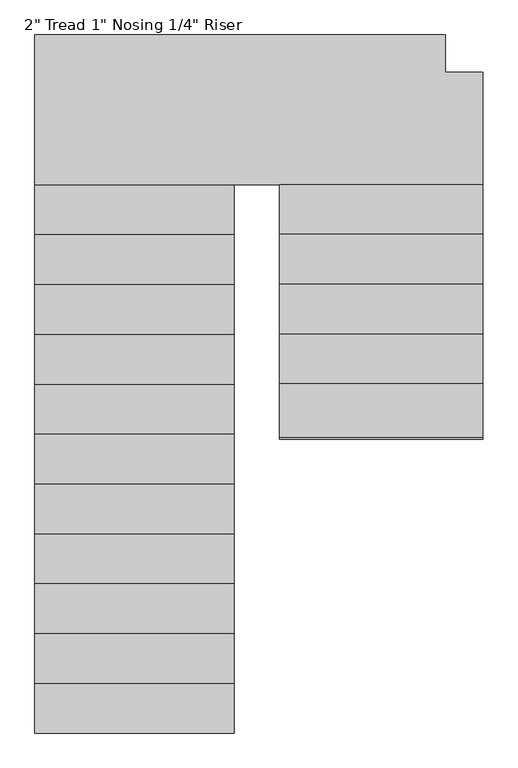
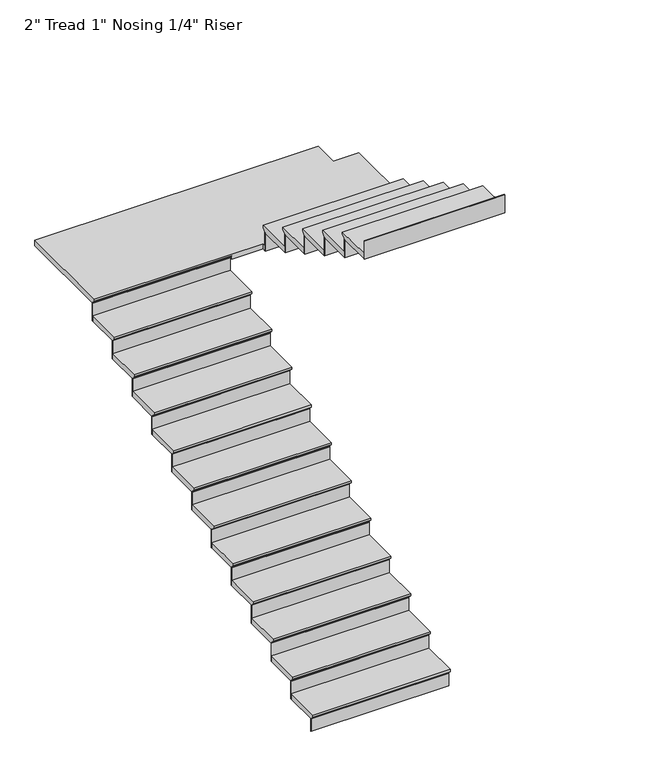
"""IFC4 building model written with IfcOpenShell, lengths in millimetres: stair flight geometry."""

from ifc_helpers import new_model, si_unit, origin, place, context, project, spatial, faceted_brep, source, transform, mapped, element, save


def stair_flight_255c1e55(model_context):
    return source(origin(), model_context, "Body", "Brep", [
        faceted_brep([(-1810.3456086, -4300.9794704, 455.0833333), (-1810.3456086, -4300.9794704, 474.1333333), (-3029.5456086, -4300.9794704, 474.1333333), (-3029.5456086, -4300.9794704, 455.0833333), (-1810.3456086, -4275.5794704, 429.6833333), (-3029.5456086, -4275.5794704, 429.6833333), (-1810.3456086, -3970.7794704, 474.1333333), (-3029.5456086, -3970.7794704, 474.1333333), (-3029.5456086, -4275.5794704, 423.3333333), (-3029.5456086, -3970.7794704, 423.3333333), (-1810.3456086, -3970.7794704, 423.3333333), (-1810.3456086, -4275.5794704, 423.3333333)], [[[0, 1, 2, 3]], [[4, 0, 3, 5]], [[2, 1, 6, 7]], [[8, 9, 10, 11]], [[2, 7, 9, 8, 5, 3]], [[8, 11, 4, 5]], [[6, 1, 0, 4, 11, 10]], [[7, 6, 10, 9]]]),
        faceted_brep([(-1810.3456086, -4275.5794704, 423.3333333), (-1810.3456086, -4275.5794704, 304.8), (-1810.3456086, -4269.2294704, 304.8), (-1810.3456086, -4269.2294704, 423.3333333), (-3029.5456086, -4275.5794704, 423.3333333), (-3029.5456086, -4269.2294704, 423.3333333), (-3029.5456086, -4269.2294704, 304.8), (-3029.5456086, -4275.5794704, 304.8)], [[[0, 1, 2, 3]], [[4, 5, 6, 7]], [[1, 0, 4, 7]], [[2, 1, 7, 6]], [[3, 2, 6, 5]], [[0, 3, 5, 4]]]),
        faceted_brep([(-1810.3456086, -3970.7794704, 592.6666667), (-1810.3456086, -3970.7794704, 423.3333333), (-1810.3456086, -3964.4294704, 423.3333333), (-1810.3456086, -3964.4294704, 592.6666667), (-3029.5456086, -3970.7794704, 592.6666667), (-3029.5456086, -3964.4294704, 592.6666667), (-3029.5456086, -3964.4294704, 423.3333333), (-3029.5456086, -3970.7794704, 423.3333333)], [[[0, 1, 2, 3]], [[4, 5, 6, 7]], [[1, 0, 4, 7]], [[2, 1, 7, 6]], [[3, 2, 6, 5]], [[0, 3, 5, 4]]]),
        faceted_brep([(-3029.5456086, -3996.1794704, 643.4666667), (-1810.3456086, -3996.1794704, 643.4666667), (-1810.3456086, -3665.9794704, 643.4666667), (-3029.5456086, -3665.9794704, 643.4666667), (-3029.5456086, -3970.7794704, 592.6666667), (-3029.5456086, -3665.9794704, 592.6666667), (-1810.3456086, -3665.9794704, 592.6666667), (-1810.3456086, -3970.7794704, 592.6666667), (-3029.5456086, -3970.7794704, 599.0166667), (-3029.5456086, -3996.1794704, 624.4166667), (-1810.3456086, -3970.7794704, 599.0166667), (-1810.3456086, -3996.1794704, 624.4166667)], [[[0, 1, 2, 3]], [[4, 5, 6, 7]], [[0, 3, 5, 4, 8, 9]], [[4, 7, 10, 8]], [[2, 1, 11, 10, 7, 6]], [[3, 2, 6, 5]], [[11, 1, 0, 9]], [[10, 11, 9, 8]]]),
        faceted_brep([(-1810.3456086, -3665.9794704, 762.0), (-1810.3456086, -3665.9794704, 592.6666667), (-1810.3456086, -3659.6294704, 592.6666667), (-1810.3456086, -3659.6294704, 762.0), (-3029.5456086, -3665.9794704, 762.0), (-3029.5456086, -3659.6294704, 762.0), (-3029.5456086, -3659.6294704, 592.6666667), (-3029.5456086, -3665.9794704, 592.6666667)], [[[0, 1, 2, 3]], [[4, 5, 6, 7]], [[1, 0, 4, 7]], [[2, 1, 7, 6]], [[3, 2, 6, 5]], [[0, 3, 5, 4]]]),
        faceted_brep([(-3029.5456086, -3691.3794704, 812.8), (-1810.3456086, -3691.3794704, 812.8), (-1810.3456086, -3361.1794704, 812.8), (-3029.5456086, -3361.1794704, 812.8), (-3029.5456086, -3665.9794704, 762.0), (-3029.5456086, -3361.1794704, 762.0), (-1810.3456086, -3361.1794704, 762.0), (-1810.3456086, -3665.9794704, 762.0), (-3029.5456086, -3665.9794704, 768.35), (-3029.5456086, -3691.3794704, 793.75), (-1810.3456086, -3665.9794704, 768.35), (-1810.3456086, -3691.3794704, 793.75)], [[[0, 1, 2, 3]], [[4, 5, 6, 7]], [[0, 3, 5, 4, 8, 9]], [[4, 7, 10, 8]], [[2, 1, 11, 10, 7, 6]], [[3, 2, 6, 5]], [[11, 1, 0, 9]], [[10, 11, 9, 8]]]),
        faceted_brep([(-1810.3456086, -3361.1794704, 931.3333333), (-1810.3456086, -3361.1794704, 762.0), (-1810.3456086, -3354.8294704, 762.0), (-1810.3456086, -3354.8294704, 931.3333333), (-3029.5456086, -3361.1794704, 931.3333333), (-3029.5456086, -3354.8294704, 931.3333333), (-3029.5456086, -3354.8294704, 762.0), (-3029.5456086, -3361.1794704, 762.0)], [[[0, 1, 2, 3]], [[4, 5, 6, 7]], [[1, 0, 4, 7]], [[2, 1, 7, 6]], [[3, 2, 6, 5]], [[0, 3, 5, 4]]]),
        faceted_brep([(-3029.5456086, -3386.5794704, 982.1333333), (-1810.3456086, -3386.5794704, 982.1333333), (-1810.3456086, -3056.3794704, 982.1333333), (-3029.5456086, -3056.3794704, 982.1333333), (-3029.5456086, -3361.1794704, 931.3333333), (-3029.5456086, -3056.3794704, 931.3333333), (-1810.3456086, -3056.3794704, 931.3333333), (-1810.3456086, -3361.1794704, 931.3333333), (-3029.5456086, -3361.1794704, 937.6833333), (-3029.5456086, -3386.5794704, 963.0833333), (-1810.3456086, -3361.1794704, 937.6833333), (-1810.3456086, -3386.5794704, 963.0833333)], [[[0, 1, 2, 3]], [[4, 5, 6, 7]], [[0, 3, 5, 4, 8, 9]], [[4, 7, 10, 8]], [[2, 1, 11, 10, 7, 6]], [[3, 2, 6, 5]], [[11, 1, 0, 9]], [[10, 11, 9, 8]]]),
        faceted_brep([(-1810.3456086, -3056.3794704, 1100.6666667), (-1810.3456086, -3056.3794704, 931.3333333), (-1810.3456086, -3050.0294704, 931.3333333), (-1810.3456086, -3050.0294704, 1100.6666667), (-3029.5456086, -3056.3794704, 1100.6666667), (-3029.5456086, -3050.0294704, 1100.6666667), (-3029.5456086, -3050.0294704, 931.3333333), (-3029.5456086, -3056.3794704, 931.3333333)], [[[0, 1, 2, 3]], [[4, 5, 6, 7]], [[1, 0, 4, 7]], [[2, 1, 7, 6]], [[3, 2, 6, 5]], [[0, 3, 5, 4]]]),
        faceted_brep([(-3029.5456086, -3081.7794704, 1151.4666667), (-1810.3456086, -3081.7794704, 1151.4666667), (-1810.3456086, -2751.5794704, 1151.4666667), (-3029.5456086, -2751.5794704, 1151.4666667), (-3029.5456086, -3056.3794704, 1100.6666667), (-3029.5456086, -2751.5794704, 1100.6666667), (-1810.3456086, -2751.5794704, 1100.6666667), (-1810.3456086, -3056.3794704, 1100.6666667), (-3029.5456086, -3056.3794704, 1107.0166667), (-3029.5456086, -3081.7794704, 1132.4166667), (-1810.3456086, -3056.3794704, 1107.0166667), (-1810.3456086, -3081.7794704, 1132.4166667)], [[[0, 1, 2, 3]], [[4, 5, 6, 7]], [[0, 3, 5, 4, 8, 9]], [[4, 7, 10, 8]], [[2, 1, 11, 10, 7, 6]], [[3, 2, 6, 5]], [[11, 1, 0, 9]], [[10, 11, 9, 8]]]),
        faceted_brep([(-1810.3456086, -2751.5794704, 1270.0), (-1810.3456086, -2751.5794704, 1100.6666667), (-1810.3456086, -2745.2294704, 1100.6666667), (-1810.3456086, -2745.2294704, 1270.0), (-3029.5456086, -2751.5794704, 1270.0), (-3029.5456086, -2745.2294704, 1270.0), (-3029.5456086, -2745.2294704, 1100.6666667), (-3029.5456086, -2751.5794704, 1100.6666667)], [[[0, 1, 2, 3]], [[4, 5, 6, 7]], [[1, 0, 4, 7]], [[2, 1, 7, 6]], [[3, 2, 6, 5]], [[0, 3, 5, 4]]]),
        faceted_brep([(-3029.5456086, -2776.9794704, 1320.8), (-1810.3456086, -2776.9794704, 1320.8), (-1810.3456086, -2446.7794704, 1320.8), (-3029.5456086, -2446.7794704, 1320.8), (-3029.5456086, -2751.5794704, 1270.0), (-3029.5456086, -2446.7794704, 1270.0), (-1810.3456086, -2446.7794704, 1270.0), (-1810.3456086, -2751.5794704, 1270.0), (-3029.5456086, -2751.5794704, 1276.35), (-3029.5456086, -2776.9794704, 1301.75), (-1810.3456086, -2751.5794704, 1276.35), (-1810.3456086, -2776.9794704, 1301.75)], [[[0, 1, 2, 3]], [[4, 5, 6, 7]], [[0, 3, 5, 4, 8, 9]], [[4, 7, 10, 8]], [[2, 1, 11, 10, 7, 6]], [[3, 2, 6, 5]], [[11, 1, 0, 9]], [[10, 11, 9, 8]]]),
        faceted_brep([(-1810.3456086, -2446.7794704, 1439.3333333), (-1810.3456086, -2446.7794704, 1270.0), (-1810.3456086, -2440.4294704, 1270.0), (-1810.3456086, -2440.4294704, 1439.3333333), (-3029.5456086, -2446.7794704, 1439.3333333), (-3029.5456086, -2440.4294704, 1439.3333333), (-3029.5456086, -2440.4294704, 1270.0), (-3029.5456086, -2446.7794704, 1270.0)], [[[0, 1, 2, 3]], [[4, 5, 6, 7]], [[1, 0, 4, 7]], [[2, 1, 7, 6]], [[3, 2, 6, 5]], [[0, 3, 5, 4]]]),
        faceted_brep([(-3029.5456086, -2472.1794704, 1490.1333333), (-1810.3456086, -2472.1794704, 1490.1333333), (-1810.3456086, -2141.9794704, 1490.1333333), (-3029.5456086, -2141.9794704, 1490.1333333), (-3029.5456086, -2446.7794704, 1439.3333333), (-3029.5456086, -2141.9794704, 1439.3333333), (-1810.3456086, -2141.9794704, 1439.3333333), (-1810.3456086, -2446.7794704, 1439.3333333), (-3029.5456086, -2446.7794704, 1445.6833333), (-3029.5456086, -2472.1794704, 1471.0833333), (-1810.3456086, -2446.7794704, 1445.6833333), (-1810.3456086, -2472.1794704, 1471.0833333)], [[[0, 1, 2, 3]], [[4, 5, 6, 7]], [[0, 3, 5, 4, 8, 9]], [[4, 7, 10, 8]], [[2, 1, 11, 10, 7, 6]], [[3, 2, 6, 5]], [[11, 1, 0, 9]], [[10, 11, 9, 8]]]),
        faceted_brep([(-1810.3456086, -2141.9794704, 1608.6666667), (-1810.3456086, -2141.9794704, 1439.3333333), (-1810.3456086, -2135.6294704, 1439.3333333), (-1810.3456086, -2135.6294704, 1608.6666667), (-3029.5456086, -2141.9794704, 1608.6666667), (-3029.5456086, -2135.6294704, 1608.6666667), (-3029.5456086, -2135.6294704, 1439.3333333), (-3029.5456086, -2141.9794704, 1439.3333333)], [[[0, 1, 2, 3]], [[4, 5, 6, 7]], [[1, 0, 4, 7]], [[2, 1, 7, 6]], [[3, 2, 6, 5]], [[0, 3, 5, 4]]]),
        faceted_brep([(-3029.5456086, -2167.3794704, 1659.4666667), (-1810.3456086, -2167.3794704, 1659.4666667), (-1810.3456086, -1837.1794704, 1659.4666667), (-3029.5456086, -1837.1794704, 1659.4666667), (-3029.5456086, -2141.9794704, 1608.6666667), (-3029.5456086, -1837.1794704, 1608.6666667), (-1810.3456086, -1837.1794704, 1608.6666667), (-1810.3456086, -2141.9794704, 1608.6666667), (-3029.5456086, -2141.9794704, 1615.0166667), (-3029.5456086, -2167.3794704, 1640.4166667), (-1810.3456086, -2141.9794704, 1615.0166667), (-1810.3456086, -2167.3794704, 1640.4166667)], [[[0, 1, 2, 3]], [[4, 5, 6, 7]], [[0, 3, 5, 4, 8, 9]], [[4, 7, 10, 8]], [[2, 1, 11, 10, 7, 6]], [[3, 2, 6, 5]], [[11, 1, 0, 9]], [[10, 11, 9, 8]]]),
        faceted_brep([(-1810.3456086, -1837.1794704, 1778.0), (-1810.3456086, -1837.1794704, 1608.6666667), (-1810.3456086, -1830.8294704, 1608.6666667), (-1810.3456086, -1830.8294704, 1778.0), (-3029.5456086, -1837.1794704, 1778.0), (-3029.5456086, -1830.8294704, 1778.0), (-3029.5456086, -1830.8294704, 1608.6666667), (-3029.5456086, -1837.1794704, 1608.6666667)], [[[0, 1, 2, 3]], [[4, 5, 6, 7]], [[1, 0, 4, 7]], [[2, 1, 7, 6]], [[3, 2, 6, 5]], [[0, 3, 5, 4]]]),
        faceted_brep([(-3029.5456086, -1862.5794704, 1828.8), (-1810.3456086, -1862.5794704, 1828.8), (-1810.3456086, -1532.3794704, 1828.8), (-3029.5456086, -1532.3794704, 1828.8), (-3029.5456086, -1837.1794704, 1778.0), (-3029.5456086, -1532.3794704, 1778.0), (-1810.3456086, -1532.3794704, 1778.0), (-1810.3456086, -1837.1794704, 1778.0), (-3029.5456086, -1837.1794704, 1784.35), (-3029.5456086, -1862.5794704, 1809.75), (-1810.3456086, -1837.1794704, 1784.35), (-1810.3456086, -1862.5794704, 1809.75)], [[[0, 1, 2, 3]], [[4, 5, 6, 7]], [[0, 3, 5, 4, 8, 9]], [[4, 7, 10, 8]], [[2, 1, 11, 10, 7, 6]], [[3, 2, 6, 5]], [[11, 1, 0, 9]], [[10, 11, 9, 8]]]),
        faceted_brep([(-1810.3456086, -1532.3794704, 1947.3333333), (-1810.3456086, -1532.3794704, 1778.0), (-1810.3456086, -1526.0294704, 1778.0), (-1810.3456086, -1526.0294704, 1947.3333333), (-3029.5456086, -1532.3794704, 1947.3333333), (-3029.5456086, -1526.0294704, 1947.3333333), (-3029.5456086, -1526.0294704, 1778.0), (-3029.5456086, -1532.3794704, 1778.0)], [[[0, 1, 2, 3]], [[4, 5, 6, 7]], [[1, 0, 4, 7]], [[2, 1, 7, 6]], [[3, 2, 6, 5]], [[0, 3, 5, 4]]]),
        faceted_brep([(-3029.5456086, -1557.7794704, 1998.1333333), (-1810.3456086, -1557.7794704, 1998.1333333), (-1810.3456086, -1227.5794704, 1998.1333333), (-3029.5456086, -1227.5794704, 1998.1333333), (-3029.5456086, -1532.3794704, 1947.3333333), (-3029.5456086, -1227.5794704, 1947.3333333), (-1810.3456086, -1227.5794704, 1947.3333333), (-1810.3456086, -1532.3794704, 1947.3333333), (-3029.5456086, -1532.3794704, 1953.6833333), (-3029.5456086, -1557.7794704, 1979.0833333), (-1810.3456086, -1532.3794704, 1953.6833333), (-1810.3456086, -1557.7794704, 1979.0833333)], [[[0, 1, 2, 3]], [[4, 5, 6, 7]], [[0, 3, 5, 4, 8, 9]], [[4, 7, 10, 8]], [[2, 1, 11, 10, 7, 6]], [[3, 2, 6, 5]], [[11, 1, 0, 9]], [[10, 11, 9, 8]]]),
        faceted_brep([(-1810.3456086, -1227.5794704, 2116.6666667), (-1810.3456086, -1227.5794704, 1947.3333333), (-1810.3456086, -1221.2294704, 1947.3333333), (-1810.3456086, -1221.2294704, 2116.6666667), (-3029.5456086, -1227.5794704, 2116.6666667), (-3029.5456086, -1221.2294704, 2116.6666667), (-3029.5456086, -1221.2294704, 1947.3333333), (-3029.5456086, -1227.5794704, 1947.3333333)], [[[0, 1, 2, 3]], [[4, 5, 6, 7]], [[1, 0, 4, 7]], [[2, 1, 7, 6]], [[3, 2, 6, 5]], [[0, 3, 5, 4]]]),
        faceted_brep([(-3029.5456086, -1252.9794704, 2167.4666667), (-1810.3456086, -1252.9794704, 2167.4666667), (-1810.3456086, -922.7794704, 2167.4666667), (-3029.5456086, -922.7794704, 2167.4666667), (-3029.5456086, -1227.5794704, 2116.6666667), (-3029.5456086, -922.7794704, 2116.6666667), (-1810.3456086, -922.7794704, 2116.6666667), (-1810.3456086, -1227.5794704, 2116.6666667), (-3029.5456086, -1227.5794704, 2123.0166667), (-3029.5456086, -1252.9794704, 2148.4166667), (-1810.3456086, -1227.5794704, 2123.0166667), (-1810.3456086, -1252.9794704, 2148.4166667)], [[[0, 1, 2, 3]], [[4, 5, 6, 7]], [[0, 3, 5, 4, 8, 9]], [[4, 7, 10, 8]], [[2, 1, 11, 10, 7, 6]], [[3, 2, 6, 5]], [[11, 1, 0, 9]], [[10, 11, 9, 8]]]),
        faceted_brep([(-1810.3456086, -922.7794704, 2286.0), (-1810.3456086, -922.7794704, 2116.6666667), (-1810.3456086, -916.4294704, 2116.6666667), (-1810.3456086, -916.4294704, 2286.0), (-3029.5456086, -922.7794704, 2286.0), (-3029.5456086, -916.4294704, 2286.0), (-3029.5456086, -916.4294704, 2116.6666667), (-3029.5456086, -922.7794704, 2116.6666667)], [[[0, 1, 2, 3]], [[4, 5, 6, 7]], [[1, 0, 4, 7]], [[2, 1, 7, 6]], [[3, 2, 6, 5]], [[0, 3, 5, 4]]]),
        faceted_brep([(-289.8083398, -973.5794704, 2336.8), (-289.8083398, -262.3794704, 2336.8), (-518.4083398, -262.3794704, 2336.8), (-518.4083398, -33.7794704, 2336.8), (-3029.5456086, -33.7794704, 2336.8), (-3029.5456086, -948.1794704, 2336.8), (-1534.4083398, -948.1794704, 2336.8), (-1534.4083398, -973.5794704, 2336.8), (-289.8083398, -262.3794704, 2286.0), (-289.8083398, -973.5794704, 2286.0), (-1534.4083398, -973.5794704, 2286.0), (-1534.4083398, -948.1794704, 2286.0), (-1810.3456086, -948.1794704, 2286.0), (-1810.3456086, -922.7794704, 2286.0), (-3029.5456086, -922.7794704, 2286.0), (-3029.5456086, -33.7794704, 2286.0), (-518.4083398, -33.7794704, 2286.0), (-518.4083398, -262.3794704, 2286.0), (-3029.5456086, -922.7794704, 2292.35), (-3029.5456086, -948.1794704, 2317.75), (-1810.3456086, -922.7794704, 2292.35), (-1810.3456086, -948.1794704, 2317.75)], [[[0, 1, 2, 3, 4, 5, 6, 7]], [[8, 9, 10, 11, 12, 13, 14, 15, 16, 17]], [[1, 0, 9, 8]], [[2, 1, 8, 17]], [[3, 2, 17, 16]], [[4, 3, 16, 15]], [[5, 4, 15, 14, 18, 19]], [[14, 13, 20, 18]], [[13, 12, 21, 20]], [[6, 5, 19, 21, 12, 11]], [[7, 6, 11, 10]], [[0, 7, 10, 9]], [[19, 18, 20, 21]]]),
        faceted_brep([(-1534.4083398, -973.5794704, 2455.3333333), (-1534.4083398, -973.5794704, 2286.0), (-1534.4083398, -979.9294704, 2286.0), (-1534.4083398, -979.9294704, 2455.3333333), (-289.8083398, -973.5794704, 2455.3333333), (-289.8083398, -979.9294704, 2455.3333333), (-289.8083398, -979.9294704, 2286.0), (-289.8083398, -973.5794704, 2286.0)], [[[0, 1, 2, 3]], [[4, 5, 6, 7]], [[1, 0, 4, 7]], [[2, 1, 7, 6]], [[3, 2, 6, 5]], [[0, 3, 5, 4]]]),
        faceted_brep([(-289.8083398, -948.1794704, 2506.1333333), (-1534.4083398, -948.1794704, 2506.1333333), (-1534.4083398, -1278.3794704, 2506.1333333), (-289.8083398, -1278.3794704, 2506.1333333), (-289.8083398, -973.5794704, 2455.3333333), (-289.8083398, -1278.3794704, 2455.3333333), (-1534.4083398, -1278.3794704, 2455.3333333), (-1534.4083398, -973.5794704, 2455.3333333), (-289.8083398, -973.5794704, 2461.6833333), (-289.8083398, -948.1794704, 2487.0833333), (-1534.4083398, -973.5794704, 2461.6833333), (-1534.4083398, -948.1794704, 2487.0833333)], [[[0, 1, 2, 3]], [[4, 5, 6, 7]], [[0, 3, 5, 4, 8, 9]], [[4, 7, 10, 8]], [[2, 1, 11, 10, 7, 6]], [[3, 2, 6, 5]], [[11, 1, 0, 9]], [[10, 11, 9, 8]]]),
        faceted_brep([(-1534.4083398, -1278.3794704, 2624.6666667), (-1534.4083398, -1278.3794704, 2455.3333333), (-1534.4083398, -1284.7294704, 2455.3333333), (-1534.4083398, -1284.7294704, 2624.6666667), (-289.8083398, -1278.3794704, 2624.6666667), (-289.8083398, -1284.7294704, 2624.6666667), (-289.8083398, -1284.7294704, 2455.3333333), (-289.8083398, -1278.3794704, 2455.3333333)], [[[0, 1, 2, 3]], [[4, 5, 6, 7]], [[1, 0, 4, 7]], [[2, 1, 7, 6]], [[3, 2, 6, 5]], [[0, 3, 5, 4]]]),
        faceted_brep([(-289.8083398, -1252.9794704, 2675.4666667), (-1534.4083398, -1252.9794704, 2675.4666667), (-1534.4083398, -1583.1794704, 2675.4666667), (-289.8083398, -1583.1794704, 2675.4666667), (-289.8083398, -1278.3794704, 2624.6666667), (-289.8083398, -1583.1794704, 2624.6666667), (-1534.4083398, -1583.1794704, 2624.6666667), (-1534.4083398, -1278.3794704, 2624.6666667), (-289.8083398, -1278.3794704, 2631.0166667), (-289.8083398, -1252.9794704, 2656.4166667), (-1534.4083398, -1278.3794704, 2631.0166667), (-1534.4083398, -1252.9794704, 2656.4166667)], [[[0, 1, 2, 3]], [[4, 5, 6, 7]], [[0, 3, 5, 4, 8, 9]], [[4, 7, 10, 8]], [[2, 1, 11, 10, 7, 6]], [[3, 2, 6, 5]], [[11, 1, 0, 9]], [[10, 11, 9, 8]]]),
        faceted_brep([(-1534.4083398, -1583.1794704, 2794.0), (-1534.4083398, -1583.1794704, 2624.6666667), (-1534.4083398, -1589.5294704, 2624.6666667), (-1534.4083398, -1589.5294704, 2794.0), (-289.8083398, -1583.1794704, 2794.0), (-289.8083398, -1589.5294704, 2794.0), (-289.8083398, -1589.5294704, 2624.6666667), (-289.8083398, -1583.1794704, 2624.6666667)], [[[0, 1, 2, 3]], [[4, 5, 6, 7]], [[1, 0, 4, 7]], [[2, 1, 7, 6]], [[3, 2, 6, 5]], [[0, 3, 5, 4]]]),
        faceted_brep([(-289.8083398, -1557.7794704, 2844.8), (-1534.4083398, -1557.7794704, 2844.8), (-1534.4083398, -1887.9794704, 2844.8), (-289.8083398, -1887.9794704, 2844.8), (-289.8083398, -1583.1794704, 2794.0), (-289.8083398, -1887.9794704, 2794.0), (-1534.4083398, -1887.9794704, 2794.0), (-1534.4083398, -1583.1794704, 2794.0), (-289.8083398, -1583.1794704, 2800.35), (-289.8083398, -1557.7794704, 2825.75), (-1534.4083398, -1583.1794704, 2800.35), (-1534.4083398, -1557.7794704, 2825.75)], [[[0, 1, 2, 3]], [[4, 5, 6, 7]], [[0, 3, 5, 4, 8, 9]], [[4, 7, 10, 8]], [[2, 1, 11, 10, 7, 6]], [[3, 2, 6, 5]], [[11, 1, 0, 9]], [[10, 11, 9, 8]]]),
        faceted_brep([(-1534.4083398, -1887.9794704, 2963.3333333), (-1534.4083398, -1887.9794704, 2794.0), (-1534.4083398, -1894.3294704, 2794.0), (-1534.4083398, -1894.3294704, 2963.3333333), (-289.8083398, -1887.9794704, 2963.3333333), (-289.8083398, -1894.3294704, 2963.3333333), (-289.8083398, -1894.3294704, 2794.0), (-289.8083398, -1887.9794704, 2794.0)], [[[0, 1, 2, 3]], [[4, 5, 6, 7]], [[1, 0, 4, 7]], [[2, 1, 7, 6]], [[3, 2, 6, 5]], [[0, 3, 5, 4]]]),
        faceted_brep([(-289.8083398, -1862.5794704, 3014.1333333), (-1534.4083398, -1862.5794704, 3014.1333333), (-1534.4083398, -2192.7794704, 3014.1333333), (-289.8083398, -2192.7794704, 3014.1333333), (-289.8083398, -1887.9794704, 2963.3333333), (-289.8083398, -2192.7794704, 2963.3333333), (-1534.4083398, -2192.7794704, 2963.3333333), (-1534.4083398, -1887.9794704, 2963.3333333), (-289.8083398, -1887.9794704, 2969.6833333), (-289.8083398, -1862.5794704, 2995.0833333), (-1534.4083398, -1887.9794704, 2969.6833333), (-1534.4083398, -1862.5794704, 2995.0833333)], [[[0, 1, 2, 3]], [[4, 5, 6, 7]], [[0, 3, 5, 4, 8, 9]], [[4, 7, 10, 8]], [[2, 1, 11, 10, 7, 6]], [[3, 2, 6, 5]], [[11, 1, 0, 9]], [[10, 11, 9, 8]]]),
        faceted_brep([(-1534.4083398, -2192.7794704, 3132.6666667), (-1534.4083398, -2192.7794704, 2963.3333333), (-1534.4083398, -2199.1294704, 2963.3333333), (-1534.4083398, -2199.1294704, 3132.6666667), (-289.8083398, -2192.7794704, 3132.6666667), (-289.8083398, -2199.1294704, 3132.6666667), (-289.8083398, -2199.1294704, 2963.3333333), (-289.8083398, -2192.7794704, 2963.3333333)], [[[0, 1, 2, 3]], [[4, 5, 6, 7]], [[1, 0, 4, 7]], [[2, 1, 7, 6]], [[3, 2, 6, 5]], [[0, 3, 5, 4]]]),
        faceted_brep([(-1534.4083398, -2497.5794704, 3302.0), (-1534.4083398, -2497.5794704, 3132.6666667), (-1534.4083398, -2503.9294704, 3132.6666667), (-1534.4083398, -2503.9294704, 3302.0), (-289.8083398, -2497.5794704, 3302.0), (-289.8083398, -2503.9294704, 3302.0), (-289.8083398, -2503.9294704, 3132.6666667), (-289.8083398, -2497.5794704, 3132.6666667)], [[[0, 1, 2, 3]], [[4, 5, 6, 7]], [[1, 0, 4, 7]], [[2, 1, 7, 6]], [[3, 2, 6, 5]], [[0, 3, 5, 4]]]),
        faceted_brep([(-289.8083398, -2167.3794704, 3183.4666667), (-1534.4083398, -2167.3794704, 3183.4666667), (-1534.4083398, -2497.5794704, 3183.4666667), (-289.8083398, -2497.5794704, 3183.4666667), (-289.8083398, -2192.7794704, 3132.6666667), (-289.8083398, -2497.5794704, 3132.6666667), (-1534.4083398, -2497.5794704, 3132.6666667), (-1534.4083398, -2192.7794704, 3132.6666667), (-289.8083398, -2192.7794704, 3139.0166667), (-289.8083398, -2167.3794704, 3164.4166667), (-1534.4083398, -2192.7794704, 3139.0166667), (-1534.4083398, -2167.3794704, 3164.4166667)], [[[0, 1, 2, 3]], [[4, 5, 6, 7]], [[0, 3, 5, 4, 8, 9]], [[4, 7, 10, 8]], [[2, 1, 11, 10, 7, 6]], [[3, 2, 6, 5]], [[11, 1, 0, 9]], [[10, 11, 9, 8]]]),
    ])


if __name__ == "__main__":
    model = new_model("IFC4")
    model_context = context("Model", 3, world=origin())
    ifc_project = project(units=[si_unit("LENGTHUNIT", "METRE", prefix="MILLI")], contexts=[model_context])
    site = spatial("IfcSite", under=ifc_project)
    building = spatial("IfcBuilding", under=site)
    placement = place(None, origin())
    stair_flight_shape = stair_flight_255c1e55(model_context)
    element("IfcStairFlight", 1, ObjectType="2\" Tread 1\" Nosing 1/4\" Riser", at=placement, inside=building, context=model_context, shape_type="MappedRepresentation", body=[
        mapped(stair_flight_shape, transform((0.0, 0.0, 0.0), x_axis=(1.0, 0.0, 0.0), y_axis=(0.0, 1.0, 0.0), z_axis=(0.0, 0.0, 1.0))),
    ])
    save(model, "model.ifc")
